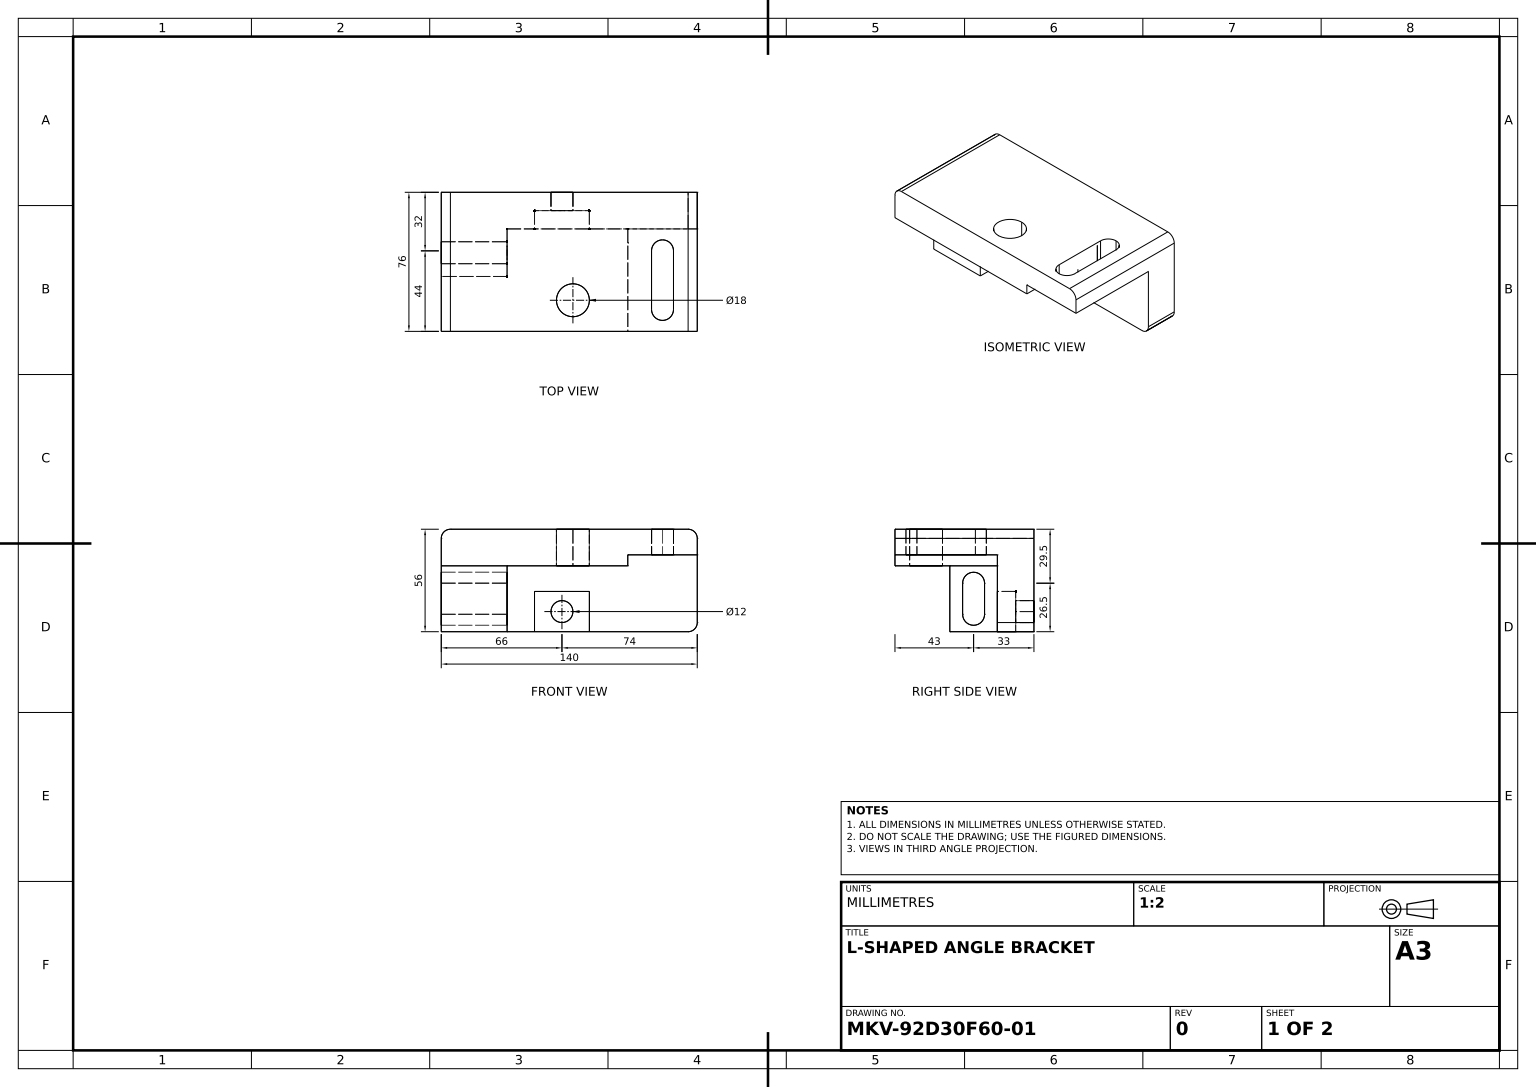
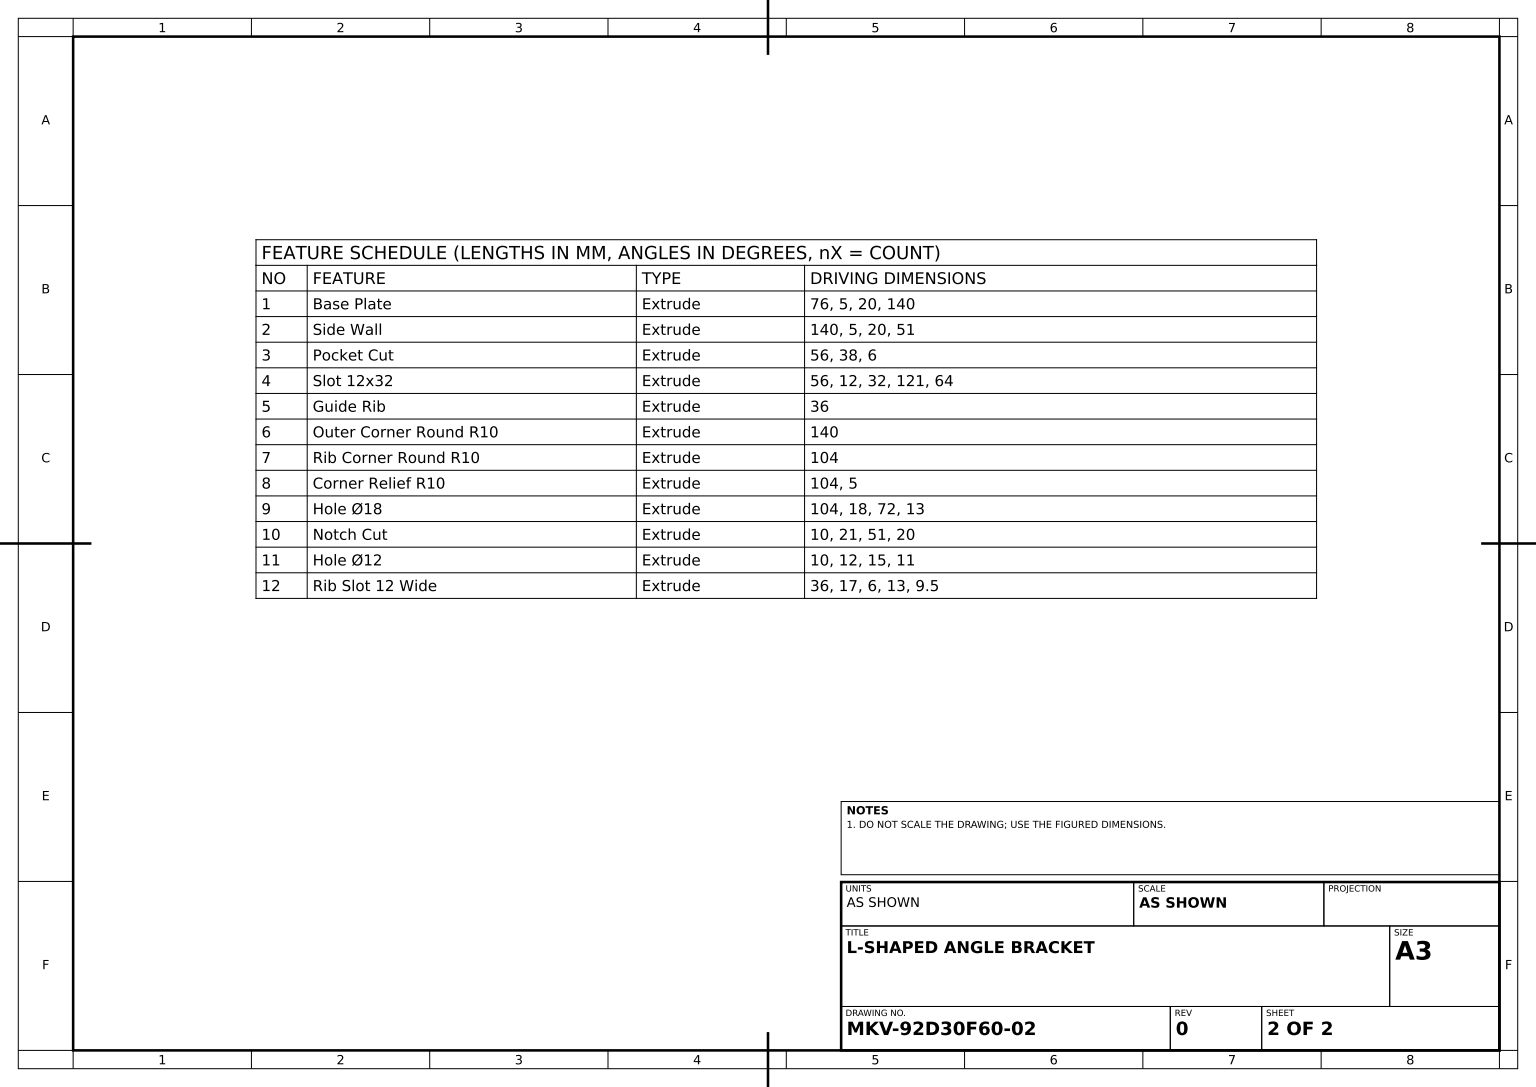
from build123d import *

# Parameters (mm, degrees)
BASE_PLATE_DEPTH             = 76
SIDE_WALL_DEPTH              = 140
POCKET_PROFILE_W             = 38
POCKET_PROFILE_H             = 6
POCKET_CUT_DEPTH             = 56
SLOT_12X32_DEPTH             = 56
GUIDE_START                  = -36
GUIDE_RIB_DEPTH              = 36
OUTER_START                  = -140
OUTER_CORNER_ROUND_R10_DEPTH = 140
RIB_CORNER_ROUND_R10_DEPTH   = 104
CORNER_RELIEF_R10_DEPTH      = 104
HOLE_18_SKETCH_R             = 9
HOLE_18_DEPTH                = 104
NOTCH_PROFILE_W              = 30
NOTCH_PROFILE_H              = 22
NOTCH_CUT_DEPTH              = 10
HOLE_12_SKETCH_R             = 6
HOLE_12_DEPTH                = 10
RIB_SLOT_12_WIDE_DEPTH       = 36


with BuildPart() as part:
    # Base Plate Profile → Base Plate (new body)
    with BuildSketch(Plane.XY):
        with BuildLine():
            Line((5, 0), (135, 0))
            ThreePointArc((135, 0), (138.535533906, -1.464466094), (140, -5))
            Line((140, -5), (140, -20))
            Line((140, -20), (0, -20))
            Line((0, -20), (0, -5))
            ThreePointArc((0, -5), (1.464466094, -1.464466094), (5, 0))
        make_face()
    extrude(amount=BASE_PLATE_DEPTH)

    # Side Wall Profile → Side Wall (add)
    with BuildSketch(Plane(origin=(140, 0, 0), x_dir=(0, 0, -1), z_dir=(1, 0, 0))):
        with BuildLine():
            Line((0, -20), (0, -51))
            ThreePointArc((0, -51), (-1.464466094, -54.535533906), (-5, -56))
            Line((-5, -56), (-15, -56))
            ThreePointArc((-15, -56), (-18.535533906, -54.535533906), (-20, -51))
            Line((-20, -51), (-20, -20))
            Line((-20, -20), (0, -20))
        make_face()
    extrude(amount=-SIDE_WALL_DEPTH)

    # Pocket Profile → Pocket Cut (cut)
    with BuildSketch(Plane.XY.offset(76)):
        with Locations((121, -17)):
            Rectangle(POCKET_PROFILE_W, POCKET_PROFILE_H)
    extrude(amount=-POCKET_CUT_DEPTH, mode=Mode.SUBTRACT)

    # Slot 12x32 Profile → Slot 12x32 (cut)
    with BuildSketch(Plane.XZ.offset(14)):
        with BuildLine():
            Line((115, 64), (115, 32))
            ThreePointArc((115, 32), (121, 26), (127, 32))
            Line((127, 32), (127, 64))
            ThreePointArc((127, 64), (121, 70), (115, 64))
        make_face()
    extrude(amount=-SLOT_12X32_DEPTH, mode=Mode.SUBTRACT)

    # Guide Rib Profile → Guide Rib (add)
    with BuildSketch(Plane.ZY.offset(GUIDE_START)):
        with BuildLine():
            Line((20, -20), (46, -20))
            Line((46, -20), (46, -56))
            Line((46, -56), (15, -56))
            ThreePointArc((15, -56), (18.535533906, -54.535533906), (20, -51))
            Line((20, -51), (20, -20))
        make_face()
    extrude(amount=GUIDE_RIB_DEPTH)

    # Outer Corner Round Profile → Outer Corner Round R10 (add)
    with BuildSketch(Plane.ZY.offset(OUTER_START)):
        with BuildLine():
            Line((0, -51), (0, -56))
            Line((0, -56), (5, -56))
            ThreePointArc((5, -56), (1.464466094, -54.535533906), (0, -51))
        make_face()
    extrude(amount=OUTER_CORNER_ROUND_R10_DEPTH)

    # Rib Corner Round Profile → Rib Corner Round R10 (add)
    with BuildSketch(Plane(origin=(140, 0, 0), x_dir=(0, 0, -1), z_dir=(1, 0, 0))):
        with BuildLine():
            Line((-20, -51), (-20, -56))
            Line((-20, -56), (-15, -56))
            ThreePointArc((-15, -56), (-18.535533906, -54.535533906), (-20, -51))
        make_face()
    extrude(amount=-RIB_CORNER_ROUND_R10_DEPTH)

    # Corner Relief Profile → Corner Relief R10 (cut)
    with BuildSketch(Plane.XY.offset(20)):
        with BuildLine():
            Line((140, -56), (140, -51))
            ThreePointArc((140, -51), (138.535533906, -54.535533906), (135, -56))
            Line((135, -56), (140, -56))
        make_face()
    extrude(amount=-CORNER_RELIEF_R10_DEPTH, mode=Mode.SUBTRACT)

    # Hole Ø18 Sketch → Hole Ø18 (cut)
    with BuildSketch(Plane.XZ.offset(20)):
        with Locations(Location((72, 59, 0), (0, 0, 270))):
            Circle(HOLE_18_SKETCH_R)
    extrude(amount=-HOLE_18_DEPTH, mode=Mode.SUBTRACT)

    # Notch Profile → Notch Cut (cut)
    with BuildSketch(Plane.XY.offset(20)):
        with Locations((66, -45)):
            Rectangle(NOTCH_PROFILE_W, NOTCH_PROFILE_H)
    extrude(amount=-NOTCH_CUT_DEPTH, mode=Mode.SUBTRACT)

    # Hole Ø12 Sketch → Hole Ø12 (cut)
    with BuildSketch(Plane.XY.offset(10)):
        with Locations((66, -45)):
            Circle(HOLE_12_SKETCH_R)
    extrude(amount=-HOLE_12_DEPTH, mode=Mode.SUBTRACT)

    # Rib Slot Profile → Rib Slot 12 Wide (cut)
    with BuildSketch(Plane(origin=(36, 0, 0), x_dir=(0, 0, -1), z_dir=(1, 0, 0))):
        with BuildLine():
            Line((-39, -29.5), (-39, -46.5))
            ThreePointArc((-39, -46.5), (-33, -52.5), (-27, -46.5))
            Line((-27, -46.5), (-27, -29.5))
            ThreePointArc((-27, -29.5), (-33, -23.5), (-39, -29.5))
        make_face()
    extrude(amount=-RIB_SLOT_12_WIDE_DEPTH, mode=Mode.SUBTRACT)


solid = part.part
